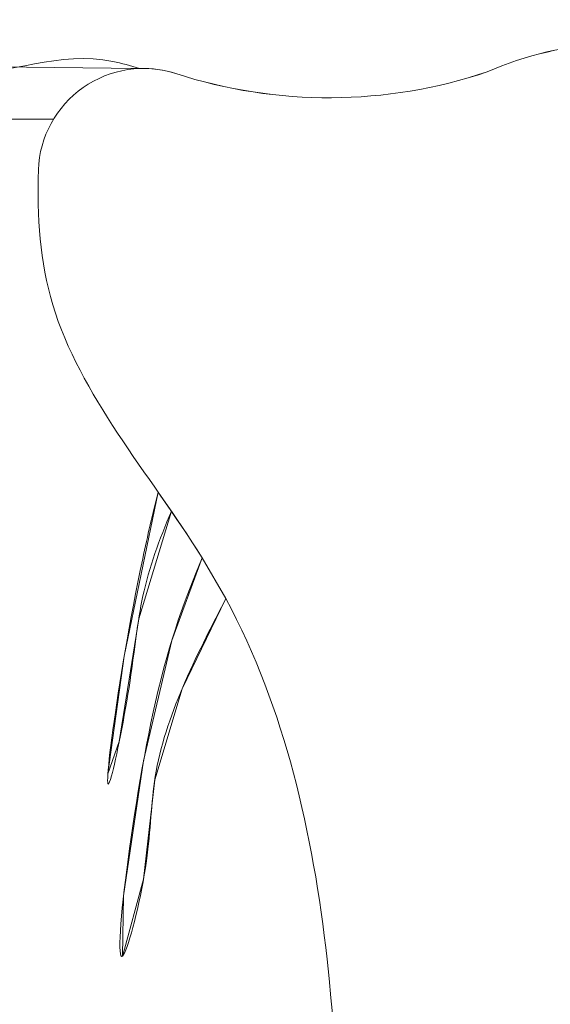
# Model space of a CAD drawing. Units: inches. Extents: x 2083 to 3317, y 1141 to 2115.
# Tile 8 of 256: x 2260 to 2278, y 1327 to 1361. Entities that reach past the tile are written whole.
import ezdxf

# ---------------------------------------------------------------- set-up
doc = ezdxf.new("R2010")
doc.units = ezdxf.units.IN
for name, color, linetype, lineweight in [('A-ANNO-DIMS', 2, 'Continuous', 18), ('A-FURN', 8, 'Continuous', 18), ('www.cadblocksfree.com', 7, 'Continuous', 9)]:
    doc.layers.add(name, color=color, linetype=linetype, lineweight=lineweight)
doc.layers.add('A-WALL-PATT', color=251, linetype='Continuous', lineweight=13, true_color=0x636466)
doc.styles.get("Standard").update_dxf_attribs({"font": 'arial.ttf'})
doc.dimstyles.new('ISO-25', dxfattribs={"dimtxt": 12, "dimasz": 12, "dimexe": 1.25, "dimexo": 0.625, "dimtad": 1, "dimlunit": 3, "dimtxsty": 'Standard', "dimcen": 2.5, "dimadec": 0, "dimazin": 0, "dimtfac": 1, "dimtmove": 0, "dimatfit": 3, "dimfxl": 1, "dimarcsym": 0})

# ---------------------------------------------------------------- blocks, each defined once
blk = doc.blocks.new('bed')
at = {"layer": 'www.cadblocksfree.com', "ltscale": 0.2}
blk.add_line((3409.943, 1443.853), (3408.408, 1442.961), dxfattribs=at)
blk.add_lwpolyline([(3426.379, 1449.413), (3426.379, 1470.154), (3363.387, 1470.154), (3363.387, 1447.076)], dxfattribs=at)
for centre, radius, start, end in [((3424.339, 1446.045), 3.937, 342.0511, 87.9851), ((3445.776, 1439.101), 18.596, 162.0511, 198.5657), ((3416.575, 1428.082), 12.646, 341.0268, 23.7782)]:
    blk.add_arc(centre, radius, start, end, dxfattribs=at)
for points, knots in [([(3428.883, 1467.22), (3428.494, 1466.08), (3427.438, 1462.983), (3429.036, 1458.154), (3427.377, 1452.621), (3429.083, 1448.872), (3428.374, 1446.522), (3428.273, 1446.192)], [0, 0, 0, 0, 0.0901802, 0.2449351, 0.3646438, 0.5132331, 0.5378548, 0.5378548, 0.5378548, 0.5378548]), ([(3409.943, 1443.853), (3413.12, 1445.837), (3417.433, 1449.66), (3422.724, 1450.042), (3424.477, 1449.98)], [1.3582378, 1.3582378, 1.3582378, 1.3582378, 1.6381418, 1.7706953, 1.7706953, 1.7706953, 1.7706953]), ([(3412.402, 1445.499), (3411.605, 1445.698), (3406.242, 1446.932), (3398.173, 1447.93), (3405.397, 1446.464), (3408.571, 1446.191), (3410.626, 1445.456), (3411.681, 1445)], [0.1043639, 0.1043639, 0.1043639, 0.1043639, 0.1489731, 0.3882761, 0.4793617, 0.5593494, 0.6446217, 0.6446217, 0.6446217, 0.6446217]), ([(3409.943, 1443.853), (3408.469, 1444.451), (3404.443, 1446.042), (3391.397, 1447.599), (3398.64, 1445.767), (3402.973, 1445.759), (3406.219, 1444.095), (3408.408, 1442.961)], [0.0056315, 0.0056315, 0.0056315, 0.0056315, 0.1489731, 0.3882761, 0.4793617, 0.5593494, 0.7397317, 0.7397317, 0.7397317, 0.7397317]), ([(3362.928, 1430.813), (3365.944, 1432.958), (3375.455, 1438.993), (3392.12, 1438.03), (3404.249, 1440.73), (3408.408, 1442.961)], [0.102872, 0.102872, 0.102872, 0.102872, 0.37972, 0.957702, 1.313793, 1.313793, 1.313793, 1.313793])]:
    blk.add_open_spline(points, degree=3, knots=knots, dxfattribs=at)
blk = doc.blocks.new('*D22')
at = {"layer": 'A-ANNO-DIMS', "color": 0, "lineweight": -2, "transparency": 16777216}
for p, q in [((2235.96, 1362.739), (2235.96, 1376.309)), ((2322.26, 1362.739), (2322.26, 1376.309)), ((2235.96, 1375.059), (2083.007, 1375.059)), ((2310.26, 1375.059), (2247.96, 1375.059))]:
    blk.add_line(p, q, dxfattribs=at)
at = {"layer": 'A-ANNO-DIMS', "color": 0, "transparency": 16777216}
for points in [[(2247.96, 1377.059), (2247.96, 1373.059), (2235.96, 1375.059)], [(2310.26, 1377.059), (2310.26, 1373.059), (2322.26, 1375.059)]]:
    blk.add_solid(points, dxfattribs=at)
at = {"layer": 'Defpoints', "color": 0, "transparency": 16777216}
for p in [(2235.96, 1375.059), (2235.96, 1362.114), (2322.26, 1362.114)]:
    blk.add_point(p, dxfattribs=at)
at = {"layer": 'A-ANNO-DIMS', "color": 0, "transparency": 16777216, "insert": (2153.483, 1381.889), "char_height": 12, "attachment_point": 5}
blk.add_mtext('BED 7\'-2 1/2" TYP.', dxfattribs=at)

msp = doc.modelspace()

# ---------------------------------------------------------------- hatches: boundary and pattern name
at = {"layer": 'A-WALL-PATT'}
h = msp.add_hatch(color=256, dxfattribs=at)
h.dxf.hatch_style = 1
h.paths.add_polyline_path([(3126.96, 2020.761), (2748.96, 2020.761), (2604.96, 2020.761), (2226.96, 2020.761), (2226.96, 1702.761), (2466.96, 1702.761), (2466.96, 1582.761), (2418.96, 1582.761), (2418.96, 1477.761), (2226.96, 1477.761), (2226.96, 1263.261), (2544.96, 1263.261), (2544.96, 1411.761), (2604.96, 1411.761), (2685.96, 1411.761), (2685.96, 1420.761), (2604.96, 1420.761), (2604.96, 1573.761), (2604.96, 1702.761), (2604.96, 2011.761), (2748.96, 2011.761), (2748.96, 1702.761), (2862.96, 1702.761), (2862.96, 1621.761), (2871.96, 1621.761), (2871.96, 1702.761), (2883.96, 1702.761), (2883.96, 1706.939, -0.026459), (2883.96, 1711.761), (2757.96, 1711.761), (2757.96, 1807.761), (2787.96, 1807.761), (2787.96, 1812.261), (2757.96, 1812.261), (2757.96, 2011.761), (2877.96, 2011.761), (2877.96, 1812.261), (2847.96, 1812.261), (2847.96, 1807.761), (2889.836, 1807.761), (2889.836, 1812.261), (2882.46, 1812.261), (2882.46, 2011.761), (3117.96, 2011.761), (3117.96, 1812.261), (2937.836, 1812.261), (2937.836, 1807.761), (2995.71, 1807.761), (2995.71, 1796.118), (3000.21, 1796.118), (3000.21, 1807.761), (3117.96, 1807.761), (3117.96, 1711.761), (3000.21, 1711.761), (3000.21, 1760.118), (2998.573, 1760.118, -0.020711), (2995.71, 1760.118), (2995.71, 1711.761), (2931.96, 1711.761), (2931.96, 1702.761), (3126.96, 1702.761)])
h.paths.add_polyline_path([(2471.46, 2011.761), (2471.46, 1810.011), (2462.717, 1810.011), (2462.717, 1805.511), (2505.96, 1805.511), (2505.96, 1810.011), (2475.96, 1810.011), (2475.96, 2011.761), (2595.96, 2011.761), (2595.96, 1810.011), (2565.96, 1810.011), (2565.96, 1805.511), (2595.96, 1805.511), (2595.96, 1711.761), (2235.96, 1711.761), (2235.96, 1805.511), (2353.71, 1805.511), (2353.71, 1796.054), (2358.21, 1796.054), (2358.21, 1805.511), (2414.717, 1805.511), (2414.717, 1810.011), (2235.96, 1810.011), (2235.96, 2011.761)], flags=16)
h.paths.add_polyline_path([(2270.205, 1994.61), (2270.205, 1970.61), (2246.205, 1970.61), (2246.205, 1994.61)], flags=0)
edge = h.paths.add_edge_path(flags=0)
edge.add_ellipse((2332.027, 1899.798), major_axis=(-3.043, 3.043), ratio=0.168252, start_angle=-161.3322, end_angle=-156.3071, ccw=False)
edge.add_ellipse((2333.082, 1898.744), major_axis=(-1.055, 1.055), ratio=0.453532, start_angle=-123.371, end_angle=-94.1591)
edge = h.paths.add_edge_path(flags=0)
edge.add_ellipse((2332.027, 1968.876), major_axis=(3.043, 3.043), ratio=0.168252, start_angle=18.6678, end_angle=23.6929)
edge.add_spline(control_points=[(2332.926, 1970.691), (2332.227, 1970.336), (2330.894, 1969.659), (2328.413, 1970.932), (2327.204, 1967.749), (2324.71, 1969.956), (2322.533, 1967.012), (2320.013, 1971.296), (2317.68, 1968.158), (2316.041, 1967.102), (2315.427, 1966.81)], knot_values=[0, 0, 0, 0, 2.267059, 4.324559, 6.685584, 8.878641, 11.121502, 14.300359, 17.755284, 19.732645, 19.732645, 19.732645, 19.732645], degree=3, periodic=0)
edge.add_ellipse((2332.027, 1968.876), major_axis=(3.043, 3.043), ratio=0.168252, start_angle=18.6678, end_angle=23.6929, ccw=False)
edge.add_ellipse((2333.082, 1969.931), major_axis=(1.055, 1.055), ratio=0.453532, start_angle=56.629, end_angle=85.8409, ccw=False)
edge = h.paths.add_edge_path(flags=0)
edge.add_spline(control_points=[(2296.428, 1967.988), (2293.628, 1965.336), (2287.704, 1959.727), (2299.744, 1949.996), (2294.533, 1935.669), (2290.573, 1920.604), (2293.394, 1909.974), (2296.185, 1904.967)], knot_values=[0.099185, 0.099185, 0.099185, 0.099185, 0.345301, 0.619822, 0.982653, 1.386093, 1.810555, 1.810555, 1.810555, 1.810555], degree=3, periodic=0)
edge.add_spline(control_points=[(2296.185, 1904.967), (2297.384, 1902.619), (2298.001, 1901.949), (2298.553, 1901.468)], knot_values=[0.006246, 0.006246, 0.006246, 0.006246, 0.055476, 0.055476, 0.055476, 0.055476], degree=3, periodic=0)
edge.add_spline(control_points=[(2298.553, 1901.468), (2297.259, 1900.923), (2295.225, 1900.232), (2293.06, 1900.614), (2292.101, 1900.788), (2292.09, 1900.791)], knot_values=[0.312835, 0.312835, 0.312835, 0.312835, 0.40178, 0.474987, 0.475903, 0.475903, 0.475903, 0.475903], degree=3, periodic=0)
edge.add_arc((2292.794, 1904.664), 3.937, 215.4209, 259.6982, ccw=False)
edge.add_spline(control_points=[(2289.585, 1902.382), (2289.477, 1902.535), (2289.368, 1902.688), (2289.261, 1902.841)], knot_values=[0.102872, 0.102872, 0.102872, 0.102872, 0.116896, 0.116896, 0.116896, 0.116896], degree=3, periodic=0)
edge.add_spline(control_points=[(2289.261, 1902.841), (2288.687, 1902.55), (2287.64, 1902.02), (2285.881, 1901.874), (2283.853, 1901.504), (2281.72, 1899.711), (2278.467, 1899.493), (2276.157, 1901.883), (2272.259, 1899.804), (2267.778, 1901.843), (2262.244, 1900.184), (2257.415, 1901.782), (2254.318, 1900.726), (2253.178, 1900.337)], knot_values=[0, 0, 0, 0, 1.907977, 3.477176, 5.261074, 7.972851, 11.680248, 13.717921, 16.939592, 22.789562, 27.502503, 33.595215, 37.145618, 37.145618, 37.145618, 37.145618], degree=3, periodic=0)
edge.add_line((2253.178, 1900.337), (2250.244, 1902.841))
edge.add_line((2250.244, 1902.841), (2250.244, 1965.833))
edge.add_line((2250.244, 1965.833), (2253.178, 1968.337))
edge.add_spline(control_points=[(2253.178, 1968.337), (2254.318, 1967.948), (2257.415, 1966.892), (2262.244, 1968.49), (2267.778, 1966.831), (2271.527, 1968.537), (2273.876, 1967.828), (2274.207, 1967.728)], knot_values=[0, 0, 0, 0, 0.09018, 0.244935, 0.364644, 0.513233, 0.537855, 0.537855, 0.537855, 0.537855], degree=3, periodic=0)
edge.add_arc((2274.353, 1963.793), 3.937, 72.0511, 92.1279, ccw=False)
edge.add_arc((2281.297, 1985.23), 18.596, 252.0511, 288.5657)
edge.add_arc((2292.317, 1956.029), 12.646, 71.0268, 113.7782, ccw=False)
edge = h.paths.add_edge_path(flags=0)
edge.add_spline(control_points=[(2274.899, 1951.856), (2275.066, 1951.617), (2275.233, 1951.377), (2275.398, 1951.136)], knot_values=[1.409916, 1.409916, 1.409916, 1.409916, 1.43159, 1.43159, 1.43159, 1.43159], degree=3, periodic=0)
edge.add_spline(control_points=[(2275.398, 1951.136), (2275.792, 1950.562), (2276.179, 1949.984), (2276.546, 1949.397)], knot_values=[1.358238, 1.358238, 1.358238, 1.358238, 1.409916, 1.409916, 1.409916, 1.409916], degree=3, periodic=0)
edge.add_line((2276.546, 1949.397), (2277.437, 1947.862))
edge.add_spline(control_points=[(2277.437, 1947.862), (2276.304, 1945.673), (2274.64, 1942.427), (2274.632, 1938.094), (2272.799, 1930.852), (2274.356, 1943.897), (2275.948, 1947.923), (2276.546, 1949.397)], knot_values=[0.005632, 0.005632, 0.005632, 0.005632, 0.186014, 0.266002, 0.357087, 0.59639, 0.739732, 0.739732, 0.739732, 0.739732], degree=3, periodic=0)
edge.add_spline(control_points=[(2276.546, 1949.397), (2276.179, 1949.984), (2275.792, 1950.562), (2275.398, 1951.136)], knot_values=[1.358238, 1.358238, 1.358238, 1.358238, 1.409916, 1.409916, 1.409916, 1.409916], degree=3, periodic=0)
edge.add_spline(control_points=[(2275.398, 1951.136), (2274.943, 1950.08), (2274.208, 1948.025), (2273.935, 1944.851), (2272.469, 1937.627), (2273.466, 1945.696), (2274.701, 1951.059), (2274.899, 1951.856)], knot_values=[0.104364, 0.104364, 0.104364, 0.104364, 0.189636, 0.269624, 0.36071, 0.600013, 0.644622, 0.644622, 0.644622, 0.644622], degree=3, periodic=0)
h.paths.add_polyline_path([(2269.168, 1963.128, -0.357527), (2268.171, 1960.976, -0.092561), (2268.171, 1939.436, -0.357527), (2269.168, 1937.285, -0.357527), (2267.016, 1938.282, -0.164785), (2254.686, 1938.282, -0.357527), (2252.534, 1937.285, -0.357527), (2253.531, 1939.436, -0.092561), (2253.531, 1960.976, -0.357527), (2252.534, 1963.128, -0.357527), (2254.686, 1962.131, -0.164785), (2267.016, 1962.131, -0.357527)], flags=0)
h.paths.add_polyline_path([(2248.874, 1967.802), (2248.874, 1957.028), (2249.458, 1957.028), (2249.458, 1911.647), (2248.874, 1911.647), (2248.874, 1900.873), (2246.512, 1900.873, 0.197327), (2244.15, 1902.457), (2244.15, 1966.218, 0.197327), (2246.512, 1967.802)], flags=0)
h.paths.add_polyline_path([(2269.168, 1931.389, -0.357527), (2268.171, 1929.238, -0.092561), (2268.171, 1907.698, -0.357527), (2269.168, 1905.547, -0.357527), (2267.016, 1906.544, -0.164785), (2254.686, 1906.544, -0.357527), (2252.534, 1905.547, -0.357527), (2253.531, 1907.698, -0.092561), (2253.531, 1929.238, -0.357527), (2252.534, 1931.389, -0.357527), (2254.686, 1930.392, -0.164785), (2267.016, 1930.392, -0.357527)], flags=0)
edge = h.paths.add_edge_path(flags=0)
edge.add_spline(control_points=[(2276.197, 1906.724), (2276.168, 1909.029), (2276.114, 1913.372), (2270.598, 1924.925), (2273.905, 1919.013), (2275.922, 1916.262), (2275.475, 1912.402), (2277.258, 1910.381), (2276.696, 1908.225), (2276.646, 1906.813), (2276.618, 1906.008)], knot_values=[0, 0, 0, 0, 8.61026, 16.221274, 18.843057, 23.804898, 27.440828, 29.356102, 31.203478, 33.650687, 33.650687, 33.650687, 33.650687], degree=3, periodic=0)
edge.add_spline(control_points=[(2276.618, 1906.008), (2276.623, 1905.624), (2276.498, 1904.629), (2275.442, 1903.855), (2274.937, 1903.08), (2274.859, 1902.841)], knot_values=[0.156488, 0.156488, 0.156488, 0.156488, 0.184398, 0.231376, 0.250598, 0.250598, 0.250598, 0.250598], degree=3, periodic=0)
edge.add_line((2274.859, 1902.841), (2276.506, 1902.841))
edge.add_spline(control_points=[(2276.506, 1902.841), (2276.788, 1903.085), (2277.665, 1904.125), (2278.25, 1904.341), (2277.654, 1908.527), (2278.156, 1906.228), (2278.1, 1905.286), (2278.847, 1904.069), (2277.857, 1903.415), (2277.874, 1902.991), (2277.904, 1902.841)], knot_values=[0.059574, 0.059574, 0.059574, 0.059574, 0.080753, 0.103741, 0.16972, 0.176036, 0.207137, 0.240474, 0.262341, 0.27366, 0.27366, 0.27366, 0.27366], degree=3, periodic=0)
edge.add_line((2277.904, 1902.841), (2280.03, 1902.841))
edge.add_spline(control_points=[(2280.03, 1902.841), (2279.888, 1903.088), (2279.499, 1903.982), (2280.152, 1905.939), (2278.104, 1909.658), (2279.762, 1907.185), (2280.328, 1904.875), (2280.485, 1903.49), (2281.463, 1903.249), (2281.758, 1902.936), (2281.834, 1902.841)], knot_values=[0.013856, 0.013856, 0.013856, 0.013856, 0.034874, 0.088867, 0.107879, 0.126738, 0.158714, 0.193757, 0.217487, 0.226722, 0.226722, 0.226722, 0.226722], degree=3, periodic=0)
edge.add_spline(control_points=[(2281.834, 1902.841), (2281.788, 1902.827), (2281.647, 1902.783), (2281.396, 1902.859), (2281.088, 1902.985), (2280.721, 1903.061), (2280.333, 1903.026), (2280.125, 1902.899), (2280.03, 1902.841)], knot_values=[0, 0, 0, 0, 0.14413, 0.435517, 0.749276, 1.153046, 1.548371, 1.878348, 1.878348, 1.878348, 1.878348], degree=3, periodic=0)
edge.add_line((2280.03, 1902.841), (2277.904, 1902.841))
edge.add_spline(control_points=[(2277.904, 1902.841), (2277.893, 1902.796), (2277.865, 1902.68), (2277.607, 1902.687), (2277.274, 1902.801), (2276.838, 1902.62), (2276.584, 1902.789), (2276.506, 1902.841)], knot_values=[0, 0, 0, 0, 0.127189, 0.326199, 0.628009, 1.24357, 1.515331, 1.515331, 1.515331, 1.515331], degree=3, periodic=0)
edge.add_line((2276.506, 1902.841), (2274.859, 1902.841))
edge.add_spline(control_points=[(2274.859, 1902.841), (2274.814, 1902.899), (2274.725, 1903.013), (2274.493, 1903.119), (2274.244, 1902.961), (2273.937, 1903.185), (2273.614, 1902.983), (2273.408, 1902.883), (2273.322, 1902.841)], knot_values=[0, 0, 0, 0, 0.21843, 0.436957, 0.687977, 0.990379, 1.398396, 1.69185, 1.69185, 1.69185, 1.69185], degree=3, periodic=0)
edge.add_spline(control_points=[(2273.322, 1902.841), (2273.617, 1903.446), (2274.274, 1904.538), (2276.027, 1904.574), (2276.207, 1906.584), (2276.197, 1906.724)], knot_values=[0.012227, 0.012227, 0.012227, 0.012227, 0.059472, 0.106218, 0.134458, 0.134458, 0.134458, 0.134458], degree=3, periodic=0)
h.paths.add_polyline_path([(2270.776, 1897.79), (2270.776, 1873.79), (2246.776, 1873.79), (2246.776, 1897.79)], flags=0)
h.paths.add_polyline_path([(2353.71, 1760.005), (2353.71, 1760.054), (2358.21, 1760.054, -0.033729)], flags=0)
h.paths.add_polyline_path([(2321.819, 1737.529), (2341.995, 1737.529, -0.414214), (2343.203, 1736.321), (2343.203, 1721.021, -0.414214), (2341.995, 1719.813), (2321.819, 1719.813, -0.414214), (2320.611, 1721.021), (2320.611, 1736.321, -0.414214)], flags=0)
h.paths.add_polyline_path([(2324.235, 1736.321), (2339.579, 1736.321, -0.414214), (2341.995, 1733.905), (2341.995, 1725.45, -0.414214), (2339.579, 1723.034), (2333.681, 1723.034), (2333.845, 1722.045, -0.870646), (2335.425, 1721.826, -0.767327), (2333.923, 1721.423), (2331.291, 1721.423, -0.767327), (2329.788, 1721.826, -0.870646), (2331.368, 1722.045), (2331.533, 1723.034), (2324.235, 1723.034, -0.414214), (2321.819, 1725.45), (2321.819, 1733.905, -0.414214)], flags=0)
h.paths.add_polyline_path([(2570.484, 1928.615), (2589.684, 1928.615), (2590.169, 1928.615), (2590.169, 1904.993), (2570.484, 1904.993)], flags=0)
h.paths.add_polyline_path([(2574.447, 1927.264, -1), (2572.829, 1927.264, -1)], flags=0)
h.paths.add_polyline_path([(2573.09, 1926.941), (2573.925, 1927.776), (2574.148, 1927.553), (2573.313, 1926.718)], flags=0)
h.paths.add_polyline_path([(2578.779, 1919.73, -1), (2571.592, 1919.73, -1)], flags=0)
h.paths.add_polyline_path([(2578.385, 1919.73, -1), (2571.985, 1919.73, -1)], flags=0)
h.paths.add_polyline_path([(2331.596, 1729.476, -1), (2333.618, 1729.476, -1)], flags=0)
h.paths.add_polyline_path([(2578.034, 1927.264, -1), (2576.416, 1927.264, -1)], flags=0)
h.paths.add_polyline_path([(2576.689, 1927.531), (2576.912, 1927.754), (2577.747, 1926.919), (2577.524, 1926.696)], flags=0)
h.paths.add_polyline_path([(2578.139, 1909.86, -1), (2572.232, 1909.86, -1)], flags=0)
h.paths.add_polyline_path([(2577.745, 1909.86, -1), (2572.625, 1909.86, -1)], flags=0)
h.paths.add_polyline_path([(2583.798, 1927.264, -1), (2582.179, 1927.264, -1)], flags=0)
h.paths.add_polyline_path([(2582.719, 1927.754), (2583.554, 1926.919), (2583.331, 1926.696), (2582.496, 1927.531)], flags=0)
h.paths.add_polyline_path([(2582.496, 1927.531), (2582.719, 1927.754), (2583.554, 1926.919), (2583.331, 1926.696)], flags=0)
h.paths.add_polyline_path([(2587.739, 1920.53, -1), (2581.832, 1920.53, -1)], flags=0)
h.paths.add_polyline_path([(2587.345, 1920.53, -1), (2582.225, 1920.53, -1)], flags=0)
h.paths.add_polyline_path([(2587.385, 1927.264, -1), (2585.766, 1927.264, -1)], flags=0)
h.paths.add_polyline_path([(2586.082, 1926.98), (2586.917, 1927.815), (2587.14, 1927.593), (2586.305, 1926.758)], flags=0)
h.paths.add_polyline_path([(2588.379, 1910.66, -1), (2581.192, 1910.66, -1)], flags=0)
h.paths.add_polyline_path([(2587.985, 1910.66, -1), (2581.585, 1910.66, -1)], flags=0)
h.paths.add_polyline_path([(2417.168, 1729.478), (2437.344, 1729.478, -0.414214), (2438.552, 1728.27), (2438.552, 1712.969, -0.414214), (2437.344, 1711.761), (2417.168, 1711.761, -0.414214), (2415.96, 1712.969), (2415.96, 1728.27, -0.414214)], flags=0)
h.paths.add_polyline_path([(2419.584, 1728.27), (2434.928, 1728.27, -0.414214), (2437.344, 1725.854), (2437.344, 1717.398, -0.414214), (2434.928, 1714.983), (2429.029, 1714.983), (2429.194, 1713.994, -0.870646), (2430.774, 1713.775, -0.767327), (2429.271, 1713.372), (2426.64, 1713.372, -0.767327), (2425.137, 1713.775, -0.870646), (2426.717, 1713.994), (2426.882, 1714.983), (2419.584, 1714.983, -0.414214), (2417.168, 1717.398), (2417.168, 1725.854, -0.414214)], flags=0)
h.paths.add_polyline_path([(2419.584, 1728.27), (2434.928, 1728.27, -0.414214), (2437.344, 1725.854), (2437.344, 1717.398, -0.414214), (2434.928, 1714.983), (2429.029, 1714.983), (2428.358, 1719.009), (2427.553, 1719.009), (2426.882, 1714.983), (2419.584, 1714.983, -0.414214), (2417.168, 1717.398), (2417.168, 1725.854, -0.414214)], flags=0)
h.paths.add_polyline_path([(2426.944, 1721.425, -1), (2428.967, 1721.425, -1)], flags=0)
h.paths.add_polyline_path([(2475.96, 1702.761), (2595.96, 1702.761), (2595.96, 1582.761), (2475.96, 1582.761)], flags=16)
h.paths.add_polyline_path([(2427.96, 1573.761), (2595.96, 1573.761), (2595.96, 1468.761), (2595.96, 1420.761), (2384.46, 1420.761), (2384.46, 1468.761), (2427.96, 1468.761)], flags=16)
h.paths.add_polyline_path([(2379.96, 1468.761), (2379.96, 1420.761), (2235.96, 1420.761), (2235.96, 1468.761)], flags=16)
h.paths.add_polyline_path([(2317.816, 1466.696), (2337.992, 1466.696, -0.414214), (2339.2, 1465.488), (2339.2, 1450.187, -0.414214), (2337.992, 1448.979), (2317.816, 1448.979, -0.414214), (2316.608, 1450.187), (2316.608, 1465.488, -0.414214)], flags=0)
h.paths.add_polyline_path([(2320.232, 1465.488), (2335.576, 1465.488, -0.414214), (2337.992, 1463.072), (2337.992, 1454.616, -0.414214), (2335.576, 1452.2), (2329.677, 1452.2), (2329.842, 1451.212, -0.870646), (2331.422, 1450.992, -0.767327), (2329.92, 1450.59), (2327.288, 1450.59, -0.767327), (2325.785, 1450.992, -0.870646), (2327.365, 1451.212), (2327.53, 1452.2), (2320.232, 1452.2, -0.414214), (2317.816, 1454.616), (2317.816, 1463.072, -0.414214)], flags=0)
h.paths.add_polyline_path([(2320.232, 1465.488), (2335.576, 1465.488, -0.414214), (2337.992, 1463.072), (2337.992, 1454.616, -0.414214), (2335.576, 1452.2), (2329.677, 1452.2), (2329.006, 1456.227), (2328.201, 1456.227), (2327.53, 1452.2), (2320.232, 1452.2, -0.414214), (2317.816, 1454.616), (2317.816, 1463.072, -0.414214)], flags=0)
h.paths.add_polyline_path([(2327.593, 1458.643, -1), (2329.615, 1458.643, -1)], flags=0)
h.paths.add_polyline_path([(2244.412, 1433.34), (2241.921, 1433.34, -0.414214), (2240.018, 1435.244), (2240.018, 1440.953, -0.414211), (2241.921, 1442.856), (2244.412, 1442.856, -1.976472)], flags=0)
h.paths.add_polyline_path([(2245.357, 1434.398, -0.414214), (2245.357, 1441.799, -2.144098)], flags=0)
h.paths.add_polyline_path([(2535.96, 1416.261), (2535.96, 1272.261), (2235.96, 1272.261), (2235.96, 1416.261)], flags=16)
h.paths.add_polyline_path([(2260.12, 1384.293), (2260.12, 1362.039), (2237.865, 1362.039), (2237.865, 1384.293)], flags=0)
edge = h.paths.add_edge_path(flags=0)
edge.add_line((2318.252, 1362.093), (2318.146, 1362.001))
edge.add_ellipse((2317.445, 1360.431), major_axis=(2.822, 2.822), ratio=0.168252, start_angle=18.6678, end_angle=20.9481, ccw=False)
edge.add_ellipse((2318.423, 1361.409), major_axis=(0.978, 0.978), ratio=0.453532, start_angle=56.629, end_angle=70.2262, ccw=False)
edge = h.paths.add_edge_path(flags=0)
edge.add_line((2319.107, 1295.571), (2319.015, 1295.677))
edge.add_ellipse((2317.445, 1296.378), major_axis=(-2.822, 2.822), ratio=0.168252, start_angle=-161.3322, end_angle=-159.0519, ccw=False)
edge.add_ellipse((2318.423, 1295.4), major_axis=(-0.978, 0.978), ratio=0.453532, start_angle=-123.371, end_angle=-109.7738)
edge = h.paths.add_edge_path(flags=0)
edge.add_spline(control_points=[(2284.21, 1301.17), (2284.581, 1300.445), (2284.891, 1299.892), (2285.16, 1299.461)], knot_values=[0.039066, 0.039066, 0.039066, 0.039066, 0.055476, 0.055476, 0.055476, 0.055476], degree=3, periodic=0)
edge.add_line((2285.16, 1299.461), (2284.21, 1301.17))
edge = h.paths.add_edge_path(flags=0)
edge.add_line((2280.412, 1297.298), (2283.37, 1297.036))
edge.add_line((2283.37, 1297.036), (2286.406, 1297.926))
edge.add_spline(control_points=[(2286.406, 1297.926), (2285.305, 1297.463), (2284.345, 1297.129), (2283.37, 1297.036)], knot_values=[0.394369, 0.394369, 0.394369, 0.394369, 0.475903, 0.475903, 0.475903, 0.475903], degree=3, periodic=0)
edge.add_spline(control_points=[(2283.37, 1297.036), (2283.281, 1297.028), (2282.316, 1296.957), (2281.313, 1297.134), (2280.423, 1297.296), (2280.412, 1297.298)], knot_values=[0.312835, 0.312835, 0.312835, 0.312835, 0.320246, 0.393453, 0.394369, 0.394369, 0.394369, 0.394369], degree=3, periodic=0)
edge = h.paths.add_edge_path(flags=0)
edge.add_line((2284.436, 1359.607), (2280.446, 1355.328))
edge.add_line((2280.446, 1355.328), (2279.58, 1351.018))
edge.add_line((2279.58, 1351.018), (2282.413, 1346.58))
edge.add_spline(control_points=[(2282.413, 1346.58), (2283.153, 1345.589), (2284.253, 1344.029), (2284.801, 1342.387), (2284.935, 1341.806)], knot_values=[1.240098, 1.240098, 1.240098, 1.240098, 1.332892, 1.382712, 1.382712, 1.382712, 1.382712], degree=3, periodic=0)
edge.add_spline(control_points=[(2284.935, 1341.806), (2285.319, 1340.141), (2285.233, 1338.409), (2284.91, 1336.654)], knot_values=[1.097484, 1.097484, 1.097484, 1.097484, 1.240098, 1.240098, 1.240098, 1.240098], degree=3, periodic=0)
edge.add_spline(control_points=[(2284.91, 1336.654), (2284.587, 1334.899), (2284.027, 1333.12), (2283.463, 1331.361)], knot_values=[0.95487, 0.95487, 0.95487, 0.95487, 1.097484, 1.097484, 1.097484, 1.097484], degree=3, periodic=0)
edge.add_line((2283.463, 1331.361), (2281.89, 1326.153))
edge.add_line((2281.89, 1326.153), (2280.756, 1321.056))
edge.add_line((2280.756, 1321.056), (2280.299, 1316.002))
edge.add_line((2280.299, 1316.002), (2280.716, 1310.95))
edge.add_line((2280.716, 1310.95), (2282.028, 1305.972))
edge.add_line((2282.028, 1305.972), (2284.21, 1301.17))
edge.add_spline(control_points=[(2284.21, 1301.17), (2283.341, 1302.73), (2282.612, 1304.336), (2282.028, 1305.972)], knot_values=[0.099185, 0.099185, 0.099185, 0.099185, 0.241799, 0.241799, 0.241799, 0.241799], degree=3, periodic=0)
edge.add_spline(control_points=[(2282.028, 1305.972), (2281.444, 1307.608), (2281.005, 1309.273), (2280.716, 1310.95)], knot_values=[0.241799, 0.241799, 0.241799, 0.241799, 0.384413, 0.384413, 0.384413, 0.384413], degree=3, periodic=0)
edge.add_spline(control_points=[(2280.716, 1310.95), (2280.433, 1312.588), (2280.289, 1314.277), (2280.299, 1315.962), (2280.299, 1316.002)], knot_values=[0.384413, 0.384413, 0.384413, 0.384413, 0.523647, 0.527028, 0.527028, 0.527028, 0.527028], degree=3, periodic=0)
edge.add_spline(control_points=[(2280.299, 1316.002), (2280.312, 1317.687), (2280.478, 1319.368), (2280.756, 1321.056)], knot_values=[0.527028, 0.527028, 0.527028, 0.527028, 0.669642, 0.669642, 0.669642, 0.669642], degree=3, periodic=0)
edge.add_spline(control_points=[(2280.756, 1321.056), (2281.035, 1322.744), (2281.426, 1324.44), (2281.89, 1326.153)], knot_values=[0.669642, 0.669642, 0.669642, 0.669642, 0.812256, 0.812256, 0.812256, 0.812256], degree=3, periodic=0)
edge.add_spline(control_points=[(2281.89, 1326.153), (2282.264, 1327.533), (2282.788, 1329.262), (2283.353, 1331.018), (2283.463, 1331.361)], knot_values=[0.812256, 0.812256, 0.812256, 0.812256, 0.927087, 0.95487, 0.95487, 0.95487, 0.95487], degree=3, periodic=0)
edge.add_line((2283.463, 1331.361), (2284.91, 1336.654))
edge.add_line((2284.91, 1336.654), (2284.935, 1341.806))
edge.add_line((2284.935, 1341.806), (2282.413, 1346.58))
edge.add_spline(control_points=[(2282.413, 1346.58), (2281.275, 1348.104), (2280.078, 1349.57), (2279.58, 1351.018)], knot_values=[1.382712, 1.382712, 1.382712, 1.382712, 1.525326, 1.525326, 1.525326, 1.525326], degree=3, periodic=0)
edge.add_spline(control_points=[(2279.58, 1351.018), (2279.443, 1351.415), (2279.136, 1352.857), (2279.735, 1354.29), (2280.446, 1355.328)], knot_values=[1.525326, 1.525326, 1.525326, 1.525326, 1.564439, 1.667941, 1.667941, 1.667941, 1.667941], degree=3, periodic=0)
edge.add_spline(control_points=[(2280.446, 1355.328), (2281.426, 1356.758), (2282.931, 1358.183), (2284.436, 1359.607)], knot_values=[1.667941, 1.667941, 1.667941, 1.667941, 1.810555, 1.810555, 1.810555, 1.810555], degree=3, periodic=0)
edge.add_arc((2280.623, 1348.518), 11.726, 71.0268, 113.7782)
edge.add_arc((2270.405, 1375.595), 17.244, 252.0511, 288.5657, ccw=False)
edge.add_arc((2263.966, 1355.718), 3.651, 72.0511, 92.1279)
edge.add_arc((2263.966, 1355.718), 3.651, 92.1279, 177.9851)
edge.add_spline(control_points=[(2260.318, 1355.846), (2260.26, 1354.221), (2260.551, 1350.187), (2262.999, 1346.766), (2264.473, 1344.649)], knot_values=[1.43159, 1.43159, 1.43159, 1.43159, 1.564144, 1.770695, 1.770695, 1.770695, 1.770695], degree=3, periodic=0)
edge.add_line((2264.473, 1344.649), (2264.936, 1343.983))
edge.add_spline(control_points=[(2263.801, 1340.248), (2263.843, 1340.514), (2264.067, 1341.756), (2264.513, 1343.002), (2264.935, 1343.981)], knot_values=[0.53657, 0.53657, 0.53657, 0.53657, 0.559349, 0.644622, 0.644622, 0.644622, 0.644622], degree=3, periodic=0)
edge.add_spline(control_points=[(2264.935, 1343.981), (2265.118, 1343.715), (2265.299, 1343.448), (2265.477, 1343.179)], knot_values=[1.384077, 1.384077, 1.384077, 1.384077, 1.409916, 1.409916, 1.409916, 1.409916], degree=3, periodic=0)
edge.add_spline(control_points=[(2265.477, 1343.179), (2265.655, 1342.911), (2265.829, 1342.641), (2265.999, 1342.369)], knot_values=[1.358238, 1.358238, 1.358238, 1.358238, 1.384077, 1.384077, 1.384077, 1.384077], degree=3, periodic=0)
edge.add_line((2265.999, 1342.369), (2266.826, 1340.946))
edge.add_spline(control_points=[(2266.826, 1340.946), (2268.894, 1337.09), (2271.398, 1325.843), (2270.516, 1310.569), (2275.919, 1301.861), (2277.79, 1299.199)], knot_values=[0.116896, 0.116896, 0.116896, 0.116896, 0.472987, 1.050969, 1.313793, 1.313793, 1.313793, 1.313793], degree=3, periodic=0)
edge.add_spline(control_points=[(2277.79, 1299.199), (2277.839, 1299.128), (2277.889, 1299.057), (2277.94, 1298.987)], knot_values=[0.109884, 0.109884, 0.109884, 0.109884, 0.116896, 0.116896, 0.116896, 0.116896], degree=3, periodic=0)
edge.add_line((2277.94, 1298.987), (2277.789, 1299.199))
edge.add_spline(control_points=[(2277.789, 1299.199), (2277.257, 1298.929), (2276.286, 1298.438), (2275.039, 1298.334), (2274.383, 1298.239), (2274.215, 1298.209)], knot_values=[33.12187, 33.12187, 33.12187, 33.12187, 35.029056, 36.598255, 37.144827, 37.144827, 37.144827, 37.144827], degree=3, periodic=0)
edge.add_line((2274.215, 1298.209), (2273.073, 1297.893))
edge.add_spline(control_points=[(2273.073, 1297.893), (2272.323, 1297.58), (2271.039, 1296.511), (2269.248, 1296.226), (2268.423, 1296.375)], knot_values=[26.532584, 26.532584, 26.532584, 26.532584, 29.198919, 31.839101, 31.839101, 31.839101, 31.839101], degree=3, periodic=0)
edge.add_line((2268.423, 1296.375), (2263.879, 1297.458))
edge.add_spline(control_points=[(2263.879, 1297.458), (2263.556, 1297.359), (2261.86, 1296.839), (2260.239, 1297.282), (2258.933, 1297.516)], knot_values=[15.919551, 15.919551, 15.919551, 15.919551, 16.939592, 21.226067, 21.226067, 21.226067, 21.226067], degree=3, periodic=0)
edge.add_line((2258.933, 1297.516), (2254.055, 1297.329))
edge.add_spline(control_points=[(2254.055, 1297.329), (2253.756, 1297.296), (2252.114, 1297.165), (2250.462, 1297.544), (2249.13, 1297.668)], knot_values=[5.306517, 5.306517, 5.306517, 5.306517, 6.276435, 10.613034, 10.613034, 10.613034, 10.613034], degree=3, periodic=0)
edge.add_line((2249.13, 1297.668), (2244.332, 1296.878))
edge.add_line((2244.332, 1296.878), (2241.611, 1299.199))
edge.add_line((2241.611, 1299.199), (2241.611, 1357.609))
edge.add_line((2241.611, 1357.609), (2244.332, 1359.931))
edge.add_line((2244.332, 1359.931), (2252.729, 1359.543))
edge.add_spline(control_points=[(2252.729, 1359.543), (2252.871, 1359.546), (2253.306, 1359.548), (2253.74, 1359.514), (2254.032, 1359.482)], knot_values=[0.233291, 0.233291, 0.233291, 0.233291, 0.244935, 0.268927, 0.268927, 0.268927, 0.268927], degree=3, periodic=0)
edge.add_line((2254.032, 1359.482), (2259.587, 1359.416))
edge.add_spline(control_points=[(2259.587, 1359.416), (2260.677, 1359.629), (2262.073, 1359.897), (2263.524, 1359.459), (2263.83, 1359.366)], knot_values=[0.422516, 0.422516, 0.422516, 0.422516, 0.513233, 0.537855, 0.537855, 0.537855, 0.537855], degree=3, periodic=0)
edge.add_arc((2263.966, 1355.718), 3.651, 72.0511, 92.1279, ccw=False)
edge.add_arc((2270.405, 1375.595), 17.244, 252.0511, 288.5657)
edge.add_arc((2280.623, 1348.518), 11.726, 71.0268, 113.7782, ccw=False)
h.paths.add_polyline_path([(2240.341, 1359.435), (2240.341, 1349.444), (2240.882, 1349.444), (2240.882, 1307.365), (2240.341, 1307.365), (2240.341, 1297.374), (2238.15, 1297.374, 0.197327), (2235.96, 1298.843), (2235.96, 1357.966, 0.197327), (2238.15, 1359.435)], flags=0)
h.paths.add_polyline_path([(2259.158, 1355.101, -0.357527), (2258.233, 1353.106, -0.092561), (2258.233, 1333.133, -0.357527), (2259.158, 1331.138, -0.357527), (2257.163, 1332.062, -0.164785), (2245.729, 1332.062, -0.357527), (2243.735, 1331.138, -0.357527), (2244.659, 1333.133, -0.092561), (2244.659, 1353.106, -0.357527), (2243.735, 1355.101, -0.357527), (2245.729, 1354.176, -0.164785), (2257.163, 1354.176, -0.357527)], flags=0)
edge = h.paths.add_edge_path(flags=0)
edge.add_line((2265.999, 1342.369), (2266.826, 1340.946))
edge.add_line((2266.826, 1340.946), (2265.308, 1337.814))
edge.add_line((2265.308, 1337.814), (2264.358, 1334.653))
edge.add_line((2264.358, 1334.653), (2264.262, 1333.8))
edge.add_spline(control_points=[(2264.262, 1333.8), (2264.208, 1333.187), (2264.162, 1332.366), (2264.007, 1331.414), (2263.969, 1331.202)], knot_values=[0.464444, 0.464444, 0.464444, 0.464444, 0.516691, 0.531608, 0.531608, 0.531608, 0.531608], degree=3, periodic=0)
edge.add_spline(control_points=[(2263.969, 1331.202), (2263.775, 1330.119), (2263.424, 1328.791), (2263.257, 1328.531), (2263.234, 1328.515)], knot_values=[0.372682, 0.372682, 0.372682, 0.372682, 0.44885, 0.464444, 0.464444, 0.464444, 0.464444], degree=3, periodic=0)
edge.add_spline(control_points=[(2263.234, 1328.515), (2263.096, 1328.42), (2263.131, 1329.301), (2263.275, 1330.616)], knot_values=[0.280919, 0.280919, 0.280919, 0.280919, 0.372682, 0.372682, 0.372682, 0.372682], degree=3, periodic=0)
edge.add_spline(control_points=[(2263.275, 1330.616), (2263.419, 1331.93), (2263.672, 1333.677), (2263.97, 1335.315)], knot_values=[0.189157, 0.189157, 0.189157, 0.189157, 0.280919, 0.280919, 0.280919, 0.280919], degree=3, periodic=0)
edge.add_spline(control_points=[(2263.97, 1335.315), (2264.1, 1336.032), (2264.419, 1337.622), (2264.755, 1338.864), (2264.947, 1339.491)], knot_values=[0.097394, 0.097394, 0.097394, 0.097394, 0.137578, 0.189157, 0.189157, 0.189157, 0.189157], degree=3, periodic=0)
edge.add_spline(control_points=[(2264.947, 1339.491), (2265.29, 1340.606), (2265.644, 1341.494), (2265.999, 1342.369)], knot_values=[0.005632, 0.005632, 0.005632, 0.005632, 0.097394, 0.097394, 0.097394, 0.097394], degree=3, periodic=0)
h.paths.add_polyline_path([(2259.158, 1325.671, -0.357527), (2258.233, 1323.676, -0.092561), (2258.233, 1303.703, -0.357527), (2259.158, 1301.708, -0.357527), (2257.163, 1302.633, -0.164785), (2245.729, 1302.633, -0.357527), (2243.735, 1301.708, -0.357527), (2244.659, 1303.703, -0.092561), (2244.659, 1323.676, -0.357527), (2243.735, 1325.671, -0.357527), (2245.729, 1324.747, -0.164785), (2257.163, 1324.747, -0.357527)], flags=0)
edge = h.paths.add_edge_path(flags=0)
edge.add_spline(control_points=[(2261.709, 1317.311), (2261.679, 1317.418), (2261.762, 1317.389), (2262.491, 1316.09), (2262.962, 1315.301)], knot_values=[14.955861, 14.955861, 14.955861, 14.955861, 16.221274, 18.694826, 18.694826, 18.694826, 18.694826], degree=3, periodic=0)
edge.add_spline(control_points=[(2262.962, 1315.301), (2262.99, 1315.254), (2263.702, 1314.067), (2264.349, 1313.127), (2264.73, 1312.164)], knot_values=[18.694826, 18.694826, 18.694826, 18.694826, 18.843057, 22.433791, 22.433791, 22.433791, 22.433791], degree=3, periodic=0)
edge.add_spline(control_points=[(2264.73, 1312.164), (2264.876, 1311.796), (2265.177, 1310.77), (2265.143, 1309.559), (2265.248, 1308.824)], knot_values=[22.433791, 22.433791, 22.433791, 22.433791, 23.804898, 26.172756, 26.172756, 26.172756, 26.172756], degree=3, periodic=0)
edge.add_line((2265.248, 1308.824), (2265.851, 1307.172))
edge.add_spline(control_points=[(2265.851, 1307.172), (2266.065, 1306.822), (2266.384, 1306.332), (2266.424, 1305.781), (2266.42, 1305.611)], knot_values=[28.062562, 28.062562, 28.062562, 28.062562, 29.356102, 29.911721, 29.911721, 29.911721, 29.911721], degree=3, periodic=0)
edge.add_spline(control_points=[(2266.42, 1305.611), (2266.416, 1305.433), (2266.394, 1305.25), (2266.365, 1305.066)], knot_values=[29.911721, 29.911721, 29.911721, 29.911721, 30.497837, 30.497837, 30.497837, 30.497837], degree=3, periodic=0)
edge.add_line((2266.365, 1305.066), (2266.066, 1302.136))
edge.add_spline(control_points=[(2266.066, 1302.136), (2266.071, 1301.78), (2265.998, 1301.2), (2265.663, 1300.759), (2265.509, 1300.586)], knot_values=[0.156488, 0.156488, 0.156488, 0.156488, 0.184398, 0.203543, 0.203543, 0.203543, 0.203543], degree=3, periodic=0)
edge.add_line((2265.509, 1300.586), (2264.435, 1299.199))
edge.add_line((2264.435, 1299.199), (2265.962, 1299.199))
edge.add_line((2265.962, 1299.199), (2267.336, 1301.175))
edge.add_line((2267.336, 1301.175), (2267.312, 1301.986))
edge.add_spline(control_points=[(2267.312, 1301.986), (2267.261, 1302.862), (2267.16, 1303.737), (2267.271, 1303.326)], knot_values=[0.126229, 0.126229, 0.126229, 0.126229, 0.166617, 0.166617, 0.166617, 0.166617], degree=3, periodic=0)
edge.add_spline(control_points=[(2267.271, 1303.326), (2267.28, 1303.294), (2267.31, 1303.175), (2267.373, 1302.884), (2267.406, 1302.683), (2267.418, 1302.601)], knot_values=[0.166617, 0.166617, 0.166617, 0.166617, 0.16972, 0.176036, 0.180765, 0.180765, 0.180765, 0.180765], degree=3, periodic=0)
edge.add_spline(control_points=[(2267.744, 1300.988), (2267.688, 1301.151), (2267.481, 1301.657), (2267.484, 1302.145), (2267.418, 1302.601)], knot_values=[0.180765, 0.180765, 0.180765, 0.180765, 0.193767, 0.220139, 0.220139, 0.220139, 0.220139], degree=3, periodic=0)
edge.add_line((2267.418, 1302.601), (2267.744, 1300.988))
edge.add_spline(control_points=[(2267.744, 1300.988), (2267.832, 1300.732), (2267.932, 1300.31), (2267.555, 1299.975), (2267.429, 1299.829)], knot_values=[0.220139, 0.220139, 0.220139, 0.220139, 0.240474, 0.25489, 0.25489, 0.25489, 0.25489], degree=3, periodic=0)
edge.add_line((2267.429, 1299.829), (2267.258, 1299.199))
edge.add_line((2267.258, 1299.199), (2269.23, 1299.199))
edge.add_spline(control_points=[(2269.23, 1299.199), (2269.099, 1299.429), (2268.843, 1300.016), (2269.012, 1300.916), (2268.947, 1301.661)], knot_values=[0.013856, 0.013856, 0.013856, 0.013856, 0.034874, 0.067073, 0.067073, 0.067073, 0.067073], degree=3, periodic=0)
edge.add_line((2268.947, 1301.661), (2268.432, 1303.603))
edge.add_spline(control_points=[(2268.432, 1303.603), (2268.176, 1304.192), (2267.596, 1305.251), (2268.041, 1304.623), (2268.251, 1304.282)], knot_values=[0.090155, 0.090155, 0.090155, 0.090155, 0.107879, 0.120289, 0.120289, 0.120289, 0.120289], degree=3, periodic=0)
edge.add_spline(control_points=[(2268.251, 1304.282), (2268.361, 1304.105), (2269.058, 1302.918), (2269.383, 1301.59), (2269.521, 1300.776), (2269.575, 1300.556)], knot_values=[0.120289, 0.120289, 0.120289, 0.120289, 0.126738, 0.158714, 0.173506, 0.173506, 0.173506, 0.173506], degree=3, periodic=0)
edge.add_line((2269.575, 1300.556), (2270.686, 1299.421))
edge.add_spline(control_points=[(2270.686, 1299.421), (2270.767, 1299.357), (2270.838, 1299.281), (2270.903, 1299.199)], knot_values=[0.21816, 0.21816, 0.21816, 0.21816, 0.226722, 0.226722, 0.226722, 0.226722], degree=3, periodic=0)
edge.add_line((2270.937, 1299.193), (2270.903, 1299.199))
edge.add_spline(control_points=[(2270.903, 1299.199), (2270.86, 1299.186), (2270.73, 1299.146), (2270.496, 1299.216), (2270.272, 1299.308), (2270.121, 1299.348), (2270.063, 1299.36)], knot_values=[0.939174, 0.939174, 0.939174, 0.939174, 1.083304, 1.374691, 1.68845, 1.878348, 1.878348, 1.878348, 1.878348], degree=3, periodic=0)
edge.add_line((2270.063, 1299.36), (2269.23, 1299.199))
edge.add_line((2269.23, 1299.199), (2267.258, 1299.199))
edge.add_spline(control_points=[(2267.258, 1299.199), (2267.248, 1299.157), (2267.223, 1299.05), (2266.984, 1299.057), (2266.809, 1299.116), (2266.677, 1299.109), (2266.637, 1299.105)], knot_values=[0.757665, 0.757665, 0.757665, 0.757665, 0.884854, 1.083864, 1.385675, 1.515331, 1.515331, 1.515331, 1.515331], degree=3, periodic=0)
edge.add_spline(control_points=[(2266.637, 1299.105), (2266.485, 1299.089), (2266.236, 1299.017), (2266.035, 1299.151), (2265.962, 1299.199)], knot_values=[0, 0, 0, 0, 0.485905, 0.757665, 0.757665, 0.757665, 0.757665], degree=3, periodic=0)
edge.add_line((2265.962, 1299.199), (2264.435, 1299.199))
edge.add_line((2264.435, 1299.199), (2263.858, 1299.367))
edge.add_spline(control_points=[(2263.858, 1299.367), (2263.819, 1299.371), (2263.78, 1299.386), (2263.74, 1299.402)], knot_values=[0.845925, 0.845925, 0.845925, 0.845925, 0.978627, 0.978627, 0.978627, 0.978627], degree=3, periodic=0)
edge.add_line((2263.722, 1299.396), (2263.01, 1299.199))
edge.add_spline(control_points=[(2263.01, 1299.199), (2263.246, 1299.683), (2263.506, 1300.128), (2263.873, 1300.408)], knot_values=[0.012227, 0.012227, 0.012227, 0.012227, 0.052971, 0.052971, 0.052971, 0.052971], degree=3, periodic=0)
edge.add_spline(control_points=[(2263.873, 1300.408), (2263.932, 1300.453), (2264.084, 1300.553), (2264.255, 1300.624), (2264.36, 1300.665)], knot_values=[0.052971, 0.052971, 0.052971, 0.052971, 0.059472, 0.069086, 0.069086, 0.069086, 0.069086], degree=3, periodic=0)
edge.add_line((2264.36, 1300.665), (2265.142, 1301.078))
edge.add_line((2265.142, 1301.078), (2265.676, 1302.8))
edge.add_line((2265.676, 1302.8), (2265.541, 1305.704))
edge.add_line((2265.541, 1305.704), (2264.803, 1309.328))
edge.add_line((2264.803, 1309.328), (2263.041, 1314.092))
edge.add_spline(control_points=[(2263.041, 1314.092), (2262.384, 1315.671), (2261.796, 1316.998), (2261.709, 1317.311)], knot_values=[11.216896, 11.216896, 11.216896, 11.216896, 14.955861, 14.955861, 14.955861, 14.955861], degree=3, periodic=0)
h.paths.add_polyline_path([(2871.96, 1416.261), (2895.91, 1416.261), (2895.91, 1420.761), (2871.96, 1420.761), (2871.96, 1501.761), (2862.96, 1501.761), (2862.96, 1420.761), (2805.96, 1420.761), (2805.96, 1411.761), (2862.96, 1411.761), (2862.96, 1263.261), (3126.96, 1263.261), (3126.96, 1411.761), (3126.96, 1486.761), (2943.96, 1486.761), (2943.96, 1477.761), (2967.86, 1477.761), (2967.86, 1420.761), (2943.91, 1420.761), (2943.91, 1416.261), (3117.96, 1416.261), (3117.96, 1420.761), (2972.36, 1420.761), (2972.36, 1477.761), (3117.96, 1477.761), (3117.96, 1420.761), (3117.96, 1272.261), (2871.96, 1272.261)], flags=0)
h.paths.add_polyline_path([(2457.126, 1485.943), (2527.603, 1485.943), (2527.603, 1537.636), (2457.126, 1537.636)], flags=8)
h.paths.add_polyline_path([(2481.005, 1609.982), (2590.766, 1609.982), (2590.766, 1682.003), (2481.005, 1682.003)], flags=8)
h.paths.add_polyline_path([(2483.085, 1729.127), (2553.562, 1729.127), (2553.562, 1780.82), (2483.085, 1780.82)], flags=8)

# ---------------------------------------------------------------- linework, layer by layer
at = {"layer": 'A-FURN'}
for p, q in [((2254.032, 1359.482), (2263.83, 1359.366)), ((2263.298, 1338.947), (2264.473, 1344.649)), ((2264.473, 1344.649), (2264.879, 1344.064)), ((2264.879, 1344.064), (2265.477, 1343.179)), ((2264.935, 1343.981), (2263.801, 1340.248)), ((2265.477, 1343.179), (2264.935, 1343.981)), ((2265.477, 1343.179), (2265.999, 1342.369)), ((2265.999, 1342.369), (2265.477, 1343.179)), ((2264.947, 1339.491), (2265.999, 1342.369)), ((2265.999, 1342.369), (2266.826, 1340.946)), ((2266.826, 1340.946), (2265.308, 1337.814)), ((2263.801, 1340.248), (2263.125, 1335.983)), ((2263.97, 1335.315), (2264.947, 1339.491)), ((2262.731, 1334.86), (2263.298, 1338.947)), ((2265.308, 1337.814), (2264.358, 1334.653)), ((2263.125, 1335.983), (2262.731, 1334.86)), ((2263.275, 1330.616), (2263.97, 1335.315)), ((2264.358, 1334.653), (2263.969, 1331.202)), ((2263.969, 1331.202), (2263.234, 1328.515)), ((2263.234, 1328.515), (2263.275, 1330.616))]:
    msp.add_line(p, q, dxfattribs=at)
for centre, radius, start, end in [((2280.623, 1348.518), 11.726, 71.0268, 113.7782), ((2263.966, 1355.718), 3.651, 72.0511, 92.1279), ((2270.405, 1375.595), 17.244, 252.0511, 288.5657)]:
    msp.add_arc(centre, radius, start, end, dxfattribs=at)

# ---------------------------------------------------------------- block references
at = {"layer": 'A-FURN', "xscale": 0.9272580240292334, "yscale": 0.9272580240292334, "zscale": 0.9272580240292334, "rotation": 90}
msp.add_blockref('bed', (3604.823, -1819.528), dxfattribs=at)

# ---------------------------------------------------------------- dimensions: what is measured, and where the dimension line sits
at = {"layer": 'A-ANNO-DIMS'}
dim = msp.add_linear_dim(base=(2235.96, 1375.059), p1=(2322.26, 1362.114), p2=(2235.96, 1362.114), angle=180, text='BED <> TYP.', dimstyle='ISO-25', override={"dimdec": 1, "dimlfac": 1, "dimrnd": 0, "dimzin": 1, "dimdsep": 46, "dimlunit": 4, "dimfrac": 2}, dxfattribs=at)
dim.commit()
dim.dimension.update_dxf_attribs({"geometry": '*D22', "text_midpoint": (2153.483, 1381.889)})

doc.saveas('drawing.dxf')
